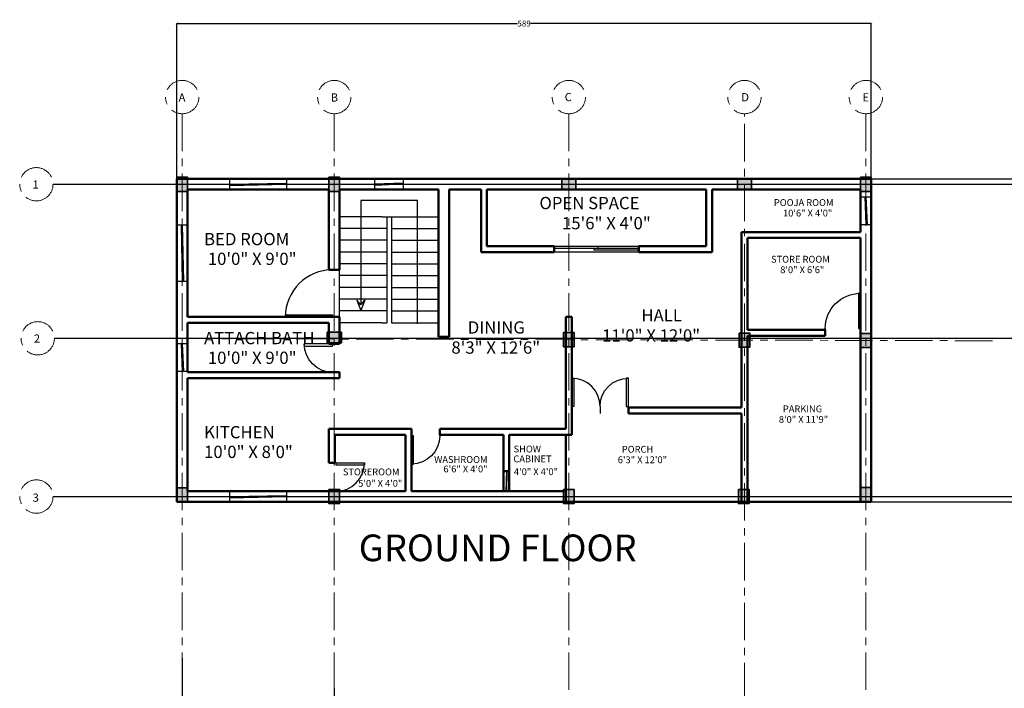
# Model space of a CAD drawing. Units: inches. Extents: x 1455 to 5994, y -182 to 2370.
# Tile 3 of 8: x 1455 to 2291, y 1803 to 2370. Entities that reach past the tile are written whole.
import ezdxf

# ---------------------------------------------------------------- set-up
doc = ezdxf.new("R2010")
doc.units = ezdxf.units.IN
doc.header["$MEASUREMENT"] = 0
doc.linetypes.add('CENTER', pattern=[50.8, 31.75, -6.35, 6.35, -6.35])
for name, color, linetype, lineweight in [('A-ANNO-DIMS', 2, 'Continuous', 18), ('A-ANNO-TEXT', 7, 'Continuous', 25), ('A-AREA-IDEN', 7, 'Continuous', 18), ('A-COLS', 7, 'Continuous', 35), ('A-COLS-PATT', 8, 'Continuous', 13), ('A-DOOR', 5, 'Continuous', 25), ('A-FLOR-STRS', 3, 'Continuous', 25), ('A-GLAZ', 4, 'Continuous', 25), ('A-GRID', 8, 'CENTER', 18), ('A-WALL', 7, 'Continuous', 50)]:
    doc.layers.add(name, color=color, linetype=linetype, lineweight=lineweight)
doc.styles.get("Standard").update_dxf_attribs({"font": 'arial.ttf'})
doc.dimstyles.get("Standard").update_dxf_attribs({"dimtxt": 5, "dimasz": 2, "dimexe": 0.18, "dimexo": 0.0625, "dimgap": 0.09, "dimtad": 0, "dimtih": 1, "dimtoh": 1, "dimdec": 1, "dimzin": 0, "dimdsep": 46, "dimlunit": 3, "dimtxsty": 'Standard', "dimblk": 'ARCHTICK', "dimcen": 0.09, "dimadec": 0, "dimazin": 0, "dimtfac": 1, "dimtdec": 1, "dimtofl": 0, "dimtmove": 0, "dimatfit": 3, "dimfxl": 1, "dimtolj": 1, "dimtzin": 0, "dimarcsym": 0})

# ---------------------------------------------------------------- blocks, each defined once
blk = doc.blocks.new('*U3')
for p, q in [((0, 0), (0, -6)), ((24, 0), (24, -6))]:
    blk.add_line(p, q)
blk.add_lwpolyline([(0, 0), (0, 24), (1.75, 24), (1.75, 0)], close=True)
blk.add_arc((0, 0), 24, 0, 90)
blk = doc.blocks.new('*U4')
for p, q in [((0, 0), (0, -6)), ((40, 0), (40, -6))]:
    blk.add_line(p, q)
blk.add_lwpolyline([(0, 0), (0, 40), (1.75, 40), (1.75, 0)], close=True)
blk.add_arc((0, 0), 40, 0, 90)
blk = doc.blocks.new('*U5')
for p, q in [((0, 0), (0, -6)), ((30, 0), (30, -6))]:
    blk.add_line(p, q)
blk.add_lwpolyline([(0, 0), (0, 30), (1.75, 30), (1.75, 0)], close=True)
blk.add_arc((0, 0), 30, 0, 90)
blk = doc.blocks.new('DOOR-SLIDING')
for p, q in [((0, 2.96), (37.51, 2.96)), ((34.07, 1.25), (34.07, 2.97)), ((72, 1.25), (34.07, 1.25)), ((37.51, 2.96), (37.51, 4.69)), ((37.51, 2.96), (72, 2.96))]:
    blk.add_line(p, q)
blk.add_lwpolyline([(0, 4.69), (72, 4.69), (72, -0.31), (0, -0.31)], close=True)
blk = doc.blocks.new('WIN-600')
for p, q in [((0, 0), (0, 24)), ((0.5, 0), (0.5, 24)), ((1, 0), (1, 24))]:
    blk.add_line(p, q)
blk = doc.blocks.new('WIN-1200')
for p, q in [((0, 1), (48, 1)), ((0, 0.5), (48, 0.5)), ((0, 0), (48, 0))]:
    blk.add_line(p, q)
blk = doc.blocks.new('WIN-450')
for p, q in [((0, 17), (0, 0)), ((0.2, 17), (0.2, 0)), ((0.4, 17), (0.4, 0))]:
    blk.add_line(p, q)
blk = doc.blocks.new('_ArchTick')
at = {"color": 0, "linetype": 'ByBlock', "const_width": 0.15}
blk.add_lwpolyline([(-0.5, -0.5), (0.5, 0.5)], dxfattribs=at)
blk = doc.blocks.new('*D35')
at = {"layer": 'A-ANNO-DIMS', "color": 0, "lineweight": -2, "transparency": 16777216}
for p, q in [((1593.29, 1828.67), (1593.29, 1744.59)), ((1722.29, 1802.99), (1722.29, 1744.59)), ((1593.29, 1744.77), (1652.41, 1744.77)), ((1722.29, 1744.77), (1663.18, 1744.77))]:
    blk.add_line(p, q, dxfattribs=at)
at = {"layer": 'Defpoints', "color": 0, "lineweight": 25, "transparency": 16777216}
for p in [(1593.29, 1828.73), (1722.29, 1803.05), (1722.29, 1744.77)]:
    blk.add_point(p, dxfattribs=at)
at = {"layer": 'A-ANNO-DIMS', "color": 0, "lineweight": -2, "transparency": 16777216, "xscale": 2, "yscale": 2, "zscale": 2, "rotation": 180}
blk.add_blockref('_ArchTick', (1593.29, 1744.77), dxfattribs=at)
at = {"layer": 'A-ANNO-DIMS', "color": 0, "lineweight": -2, "transparency": 16777216, "xscale": 2, "yscale": 2, "zscale": 2}
blk.add_blockref('_ArchTick', (1722.29, 1744.77), dxfattribs=at)
at = {"layer": 'A-ANNO-DIMS', "color": 0, "transparency": 16777216, "insert": (1657.79, 1744.77), "char_height": 5, "attachment_point": 5}
blk.add_mtext('\\A1;129', dxfattribs=at)
blk = doc.blocks.new('*D39')
at = {"layer": 'A-ANNO-DIMS', "color": 0, "lineweight": -2, "transparency": 16777216}
for p, q in [((1483.73, 2230.77), (2434.6, 2230.77)), ((2434.42, 2230.77), (2434.42, 2168.07)), ((2434.42, 2100.07), (2434.42, 2162.78)), ((1484.89, 2100.07), (2434.6, 2100.07))]:
    blk.add_line(p, q, dxfattribs=at)
at = {"layer": 'Defpoints', "color": 0, "lineweight": 25, "transparency": 16777216}
for p in [(1483.66, 2230.77), (1484.83, 2100.07), (2434.42, 2100.07)]:
    blk.add_point(p, dxfattribs=at)
at = {"layer": 'A-ANNO-DIMS', "color": 0, "lineweight": -2, "transparency": 16777216, "xscale": 2, "yscale": 2, "zscale": 2}
for p, rotation in [((2434.42, 2230.77), 90), ((2434.42, 2100.07), 270)]:
    blk.add_blockref('_ArchTick', p, dxfattribs=dict(at, rotation=rotation))
at = {"layer": 'A-ANNO-DIMS', "color": 0, "transparency": 16777216, "insert": (2434.42, 2165.42), "char_height": 5, "attachment_point": 5}
blk.add_mtext('\\A1;130.7', dxfattribs=at)
blk = doc.blocks.new('*D40')
at = {"layer": 'A-ANNO-DIMS', "color": 0, "lineweight": -2, "transparency": 16777216}
for p, q in [((1484.89, 2100.07), (2434.6, 2100.07)), ((2434.42, 2100.07), (2434.42, 2035.57)), ((2434.42, 1965.77), (2434.42, 2030.28)), ((1483.73, 1965.77), (2434.6, 1965.77))]:
    blk.add_line(p, q, dxfattribs=at)
at = {"layer": 'Defpoints', "color": 0, "lineweight": 25, "transparency": 16777216}
for p in [(1484.83, 2100.07), (1483.66, 1965.77), (2434.42, 1965.77)]:
    blk.add_point(p, dxfattribs=at)
at = {"layer": 'A-ANNO-DIMS', "color": 0, "lineweight": -2, "transparency": 16777216, "xscale": 2, "yscale": 2, "zscale": 2}
for p, rotation in [((2434.42, 2100.07), 90), ((2434.42, 1965.77), 270)]:
    blk.add_blockref('_ArchTick', p, dxfattribs=dict(at, rotation=rotation))
at = {"layer": 'A-ANNO-DIMS', "color": 0, "transparency": 16777216, "insert": (2434.42, 2032.92), "char_height": 5, "attachment_point": 5}
blk.add_mtext('\\A1;134.3', dxfattribs=at)
blk = doc.blocks.new('*D41')
at = {"layer": 'A-ANNO-DIMS', "color": 0, "lineweight": -2, "transparency": 16777216}
for p, q in [((1588.79, 2235.34), (1588.79, 2367.36)), ((1588.79, 2367.18), (1877.68, 2367.18)), ((2177.79, 2367.18), (1888.91, 2367.18)), ((2177.79, 2235.34), (2177.79, 2367.36))]:
    blk.add_line(p, q, dxfattribs=at)
at = {"layer": 'Defpoints', "color": 0, "lineweight": 25, "transparency": 16777216}
for p in [(2177.79, 2367.18), (1588.79, 2235.27), (2177.79, 2235.27)]:
    blk.add_point(p, dxfattribs=at)
at = {"layer": 'A-ANNO-DIMS', "color": 0, "lineweight": -2, "transparency": 16777216, "xscale": 2, "yscale": 2, "zscale": 2, "rotation": 180}
blk.add_blockref('_ArchTick', (1588.79, 2367.18), dxfattribs=at)
at = {"layer": 'A-ANNO-DIMS', "color": 0, "lineweight": -2, "transparency": 16777216, "xscale": 2, "yscale": 2, "zscale": 2}
blk.add_blockref('_ArchTick', (2177.79, 2367.18), dxfattribs=at)
at = {"layer": 'A-ANNO-DIMS', "color": 0, "transparency": 16777216, "insert": (1883.29, 2367.18), "char_height": 5, "attachment_point": 5}
blk.add_mtext('\\A1;589', dxfattribs=at)
blk = doc.blocks.new('*D42')
at = {"layer": 'A-ANNO-DIMS', "color": 0, "lineweight": -2, "transparency": 16777216}
for p, q in [((2177.86, 2235.27), (2434.6, 2235.27)), ((2434.42, 2235.27), (2434.42, 2100.96)), ((2434.42, 1961.36), (2434.42, 2095.67)), ((2177.86, 1961.36), (2434.6, 1961.36))]:
    blk.add_line(p, q, dxfattribs=at)
at = {"layer": 'Defpoints', "color": 0, "lineweight": 25, "transparency": 16777216}
for p in [(2177.79, 2235.27), (2434.42, 2235.27), (2177.79, 1961.36)]:
    blk.add_point(p, dxfattribs=at)
at = {"layer": 'A-ANNO-DIMS', "color": 0, "lineweight": -2, "transparency": 16777216, "xscale": 2, "yscale": 2, "zscale": 2}
for p, rotation in [((2434.42, 2235.27), 90), ((2434.42, 1961.36), 270)]:
    blk.add_blockref('_ArchTick', p, dxfattribs=dict(at, rotation=rotation))
at = {"layer": 'A-ANNO-DIMS', "color": 0, "transparency": 16777216, "insert": (2434.42, 2098.32), "char_height": 5, "attachment_point": 5}
blk.add_mtext('\\A1;273.9', dxfattribs=at)

msp = doc.modelspace()

# ---------------------------------------------------------------- hatches: boundary and pattern name
at = {"layer": 'A-COLS-PATT'}
h = msp.add_hatch(color=256, dxfattribs=at)
h.dxf.hatch_style = 1
h.paths.add_polyline_path([(1597.7942, 2236.774), (1588.7942, 2236.774), (1588.7942, 2224.774), (1597.7942, 2224.774)])
h = msp.add_hatch(color=256, dxfattribs=at)
h.dxf.hatch_style = 1
h.paths.add_polyline_path([(1726.7942, 2236.774), (1717.7942, 2236.774), (1717.7942, 2224.774), (1726.7942, 2224.774)])
h = msp.add_hatch(color=256, dxfattribs=at)
h.dxf.hatch_style = 1
h.paths.add_polyline_path([(1915.2942, 2235.274), (1915.2942, 2226.274), (1927.2942, 2226.274), (1927.2942, 2235.274)])
h = msp.add_hatch(color=256, dxfattribs=at)
h.dxf.hatch_style = 1
h.paths.add_polyline_path([(2064.2942, 2235.274), (2064.2942, 2226.274), (2076.2942, 2226.274), (2076.2942, 2235.274)])
h = msp.add_hatch(color=256, dxfattribs=at)
h.dxf.hatch_style = 1
h.paths.add_polyline_path([(2177.7942, 2236.774), (2168.7942, 2236.774), (2168.7942, 2224.774), (2177.7942, 2224.774)])
h = msp.add_hatch(color=256, dxfattribs=at)
h.dxf.hatch_style = 1
h.paths.add_polyline_path([(1716.2942, 2105.179), (1716.2942, 2096.179), (1728.2942, 2096.179), (1728.2942, 2105.179)])
h = msp.add_hatch(color=256, dxfattribs=at)
h.dxf.hatch_style = 1
h.paths.add_polyline_path([(1925.7942, 2104.9263), (1916.7942, 2104.9263), (1916.7942, 2092.9263), (1925.7942, 2092.9263)])
h = msp.add_hatch(color=256, dxfattribs=at)
h.dxf.hatch_style = 1
h.paths.add_polyline_path([(2074.7942, 2104.537), (2065.7942, 2104.537), (2065.7942, 2092.537), (2074.7942, 2092.537)])
h = msp.add_hatch(color=256, dxfattribs=at)
h.dxf.hatch_style = 1
h.paths.add_polyline_path([(2177.7942, 2104.2678), (2168.7942, 2104.2678), (2168.7942, 2092.2678), (2177.7942, 2092.2678)])
h = msp.add_hatch(color=256, dxfattribs=at)
h.dxf.hatch_style = 1
h.paths.add_polyline_path([(1597.7942, 1973.1902), (1588.7942, 1973.1902), (1588.7942, 1961.1902), (1597.7942, 1961.1902)])
h = msp.add_hatch(color=256, dxfattribs=at)
h.dxf.hatch_style = 1
h.paths.add_polyline_path([(1726.7942, 1971.774), (1717.7942, 1971.774), (1717.7942, 1959.774), (1726.7942, 1959.774)])
h = msp.add_hatch(color=256, dxfattribs=at)
h.dxf.hatch_style = 1
h.paths.add_polyline_path([(1925.7942, 1971.774), (1916.7942, 1971.774), (1916.7942, 1959.774), (1925.7942, 1959.774)])
h = msp.add_hatch(color=256, dxfattribs=at)
h.dxf.hatch_style = 1
h.paths.add_polyline_path([(2074.1779, 1971.774), (2065.1779, 1971.774), (2065.1779, 1959.774), (2074.1779, 1959.774)])
h = msp.add_hatch(color=256, dxfattribs=at)
h.dxf.hatch_style = 1
h.paths.add_polyline_path([(2177.7942, 1973.3596), (2168.7942, 1973.3596), (2168.7942, 1961.3596), (2177.7942, 1961.3596)])

# ---------------------------------------------------------------- linework, layer by layer
at = {"layer": 'A-COLS'}
for points in [[(1588.7942, 2236.774), (1597.7942, 2236.774), (1597.7942, 2224.774), (1588.7942, 2224.774)], [(1717.7942, 2236.774), (1726.7942, 2236.774), (1726.7942, 2224.774), (1717.7942, 2224.774)], [(1915.2942, 2226.274), (1915.2942, 2235.274), (1927.2942, 2235.274), (1927.2942, 2226.274)], [(2064.2942, 2226.274), (2064.2942, 2235.274), (2076.2942, 2235.274), (2076.2942, 2226.274)], [(2168.7942, 2236.774), (2177.7942, 2236.774), (2177.7942, 2224.774), (2168.7942, 2224.774)], [(1716.2942, 2096.179), (1716.2942, 2105.179), (1728.2942, 2105.179), (1728.2942, 2096.179)], [(1916.7942, 2104.9263), (1925.7942, 2104.9263), (1925.7942, 2092.9263), (1916.7942, 2092.9263)], [(2065.7942, 2104.537), (2074.7942, 2104.537), (2074.7942, 2092.537), (2065.7942, 2092.537)], [(2168.7942, 2104.2678), (2177.7942, 2104.2678), (2177.7942, 2092.2678), (2168.7942, 2092.2678)], [(1588.7942, 1973.1902), (1597.7942, 1973.1902), (1597.7942, 1961.1902), (1588.7942, 1961.1902)], [(1717.7942, 1971.774), (1726.7942, 1971.774), (1726.7942, 1959.774), (1717.7942, 1959.774)], [(1916.7942, 1971.774), (1925.7942, 1971.774), (1925.7942, 1959.774), (1916.7942, 1959.774)], [(2065.1779, 1971.774), (2074.1779, 1971.774), (2074.1779, 1959.774), (2065.1779, 1959.774)], [(2168.7942, 1973.3596), (2177.7942, 1973.3596), (2177.7942, 1961.3596), (2168.7942, 1961.3596)]]:
    msp.add_lwpolyline(points, close=True, dxfattribs=at)
at = {"layer": 'A-FLOR-STRS'}
for p, q in [((1792.7942, 2217.1453), (1744.7942, 2217.1453)), ((1744.7942, 2217.1453), (1744.7942, 2128.5876)), ((1792.7942, 2112.4497), (1792.7942, 2217.1453)), ((1762.7942, 2203.274), (1726.7942, 2203.274)), ((1762.7942, 2203.274), (1774.7942, 2203.274)), ((1766.7942, 2203.274), (1766.7942, 2113.274)), ((1770.7942, 2203.274), (1770.7942, 2113.274)), ((1774.7942, 2203.274), (1810.7942, 2203.274)), ((1766.7942, 2193.274), (1726.7942, 2193.274)), ((1770.7942, 2193.274), (1810.7942, 2193.274)), ((1766.7942, 2183.274), (1726.7942, 2183.274)), ((1770.7942, 2183.274), (1810.7942, 2183.274)), ((1766.7942, 2173.274), (1726.7942, 2173.274)), ((1770.7942, 2173.274), (1810.7942, 2173.274)), ((1766.7942, 2163.274), (1726.7942, 2163.274)), ((1726.7942, 2113.274), (1726.7942, 2160.274)), ((1770.7942, 2163.274), (1810.7942, 2163.274)), ((1766.7942, 2153.274), (1726.7942, 2153.274)), ((1770.7942, 2153.274), (1810.7942, 2153.274)), ((1766.7942, 2143.274), (1726.7942, 2143.274)), ((1770.7942, 2143.274), (1810.7942, 2143.274)), ((1766.7942, 2133.274), (1726.7942, 2133.274)), ((1744.7942, 2128.5876), (1741.4465, 2132.4497)), ((1741.4465, 2132.4497), (1744.7942, 2123.5688)), ((1744.7942, 2128.5876), (1748.1419, 2132.4497)), ((1748.1419, 2132.4497), (1744.7942, 2123.5688)), ((1770.7942, 2133.274), (1810.7942, 2133.274)), ((1766.7942, 2123.274), (1726.7942, 2123.274)), ((1770.7942, 2123.274), (1810.7942, 2123.274)), ((1762.7942, 2113.274), (1726.7942, 2113.274)), ((1762.7942, 2113.274), (1766.7942, 2113.274)), ((1770.7942, 2113.274), (1774.7942, 2113.274)), ((1774.7942, 2113.274), (1810.7942, 2113.274))]:
    msp.add_line(p, q, dxfattribs=at)
at = {"layer": 'A-GLAZ'}
for points in [[(1633.7942, 2235.274), (1681.7942, 2235.274), (1681.7942, 2226.274), (1633.7942, 2226.274)], [(1756.7942, 2235.274), (1780.7942, 2235.274), (1780.7942, 2226.274), (1756.7942, 2226.274)], [(2168.7942, 2196.274), (2168.7942, 2220.274), (2177.7942, 2220.274), (2177.7942, 2196.274)], [(1597.7942, 2196.274), (1597.7942, 2148.274), (1588.7942, 2148.274), (1588.7942, 2196.274)], [(1588.7942, 2071.7739), (1588.7942, 2095.7739), (1597.7942, 2095.7739), (1597.7942, 2071.7739)], [(1870.7942, 1970.274), (1865.7942, 1970.274), (1865.7942, 1987.274), (1870.7942, 1987.274)], [(1633.7942, 1970.274), (1681.7942, 1970.274), (1681.7942, 1961.274), (1633.7942, 1961.274)]]:
    msp.add_lwpolyline(points, close=True, dxfattribs=at)
at = {"layer": 'A-GRID'}
for p, q in [((1593.2942, 2290.6569), (1593.2942, 1828.7288)), ((1722.2942, 2290.6569), (1722.2942, 1803.0507)), ((1921.2942, 2290.6569), (1921.2942, 1801.7341)), ((2070.2942, 1793.0189), (2070.2942, 2290.6569)), ((2173.2942, 2290.6569), (2173.2942, 1794.3991)), ((1483.6636, 2230.774), (2284.5122, 2230.774)), ((2280.5998, 2097.9874), (1484.8312, 2100.0669)), ((1483.6636, 1965.774), (2386.1674, 1965.774))]:
    msp.add_line(p, q, dxfattribs=at)
for centre in [(1593.2942, 2304.7952), (1722.2942, 2304.7952), (1921.2942, 2304.7952), (2070.2942, 2304.7952), (2173.2942, 2304.7952), (1469.5253, 2230.774), (1470.6929, 2100.0669), (1469.5253, 1965.774)]:
    msp.add_circle(centre, 14.1383, dxfattribs=at)
at = {"layer": 'A-WALL'}
for p, q in [((1588.7942, 2235.274), (1588.7942, 1961.274)), ((1588.7942, 2235.274), (2177.7942, 2235.274)), ((2177.7942, 2235.274), (2177.7942, 1961.274)), ((1597.7942, 2226.274), (1597.7942, 2118.274)), ((1597.7942, 2226.274), (1717.7942, 2226.274)), ((1717.7942, 2226.274), (1717.7942, 2158.1614)), ((1726.7942, 2226.274), (1726.7942, 2158.274)), ((1726.7942, 2226.274), (1810.7942, 2226.274)), ((1810.7942, 2226.274), (1810.7942, 2101.2917)), ((1819.7942, 2226.274), (1819.7942, 2101.2917)), ((1819.7942, 2226.274), (1846.7942, 2226.274)), ((1846.7942, 2226.274), (1846.7942, 2190.274)), ((1851.7942, 2226.274), (1851.7942, 2190.274)), ((1851.7942, 2226.274), (2037.7942, 2226.274)), ((2037.7942, 2226.274), (2037.7942, 2178.274)), ((2042.7942, 2226.274), (2042.7942, 2190.274)), ((2042.7942, 2226.274), (2067.7942, 2226.274)), ((2067.7942, 2226.274), (2168.7942, 2226.274)), ((2168.7942, 2226.274), (2168.7942, 2190.274)), ((1846.7942, 2190.274), (1846.7942, 2173.274)), ((1851.7942, 2190.274), (1851.7942, 2178.274)), ((2042.7942, 2190.274), (2042.7942, 2173.274)), ((2067.7942, 2190.274), (2067.7942, 2041.274)), ((2067.7942, 2190.274), (2168.7942, 2190.274)), ((2072.7942, 2185.274), (2072.7942, 2107.274)), ((2072.7942, 2185.274), (2168.7942, 2185.274)), ((2168.7942, 2185.274), (2168.7942, 2119.274)), ((1846.7942, 2173.274), (1908.7942, 2173.274)), ((1851.7942, 2178.274), (1908.7942, 2178.274)), ((1908.7942, 2178.274), (1908.7942, 2173.274)), ((1980.7942, 2178.274), (2037.7942, 2178.274)), ((1980.7942, 2178.274), (1980.7942, 2173.274)), ((1980.7942, 2173.274), (2042.7942, 2173.274)), ((1717.7942, 2158.1614), (1726.7942, 2158.274)), ((1597.7942, 2118.274), (1717.7942, 2118.274)), ((1717.7942, 2118.274), (1726.7942, 2118.274)), ((1726.7942, 2118.274), (1726.7942, 2113.274)), ((1918.7942, 2118.274), (1918.7942, 2023.274)), ((1918.7942, 2118.274), (1923.7942, 2118.274)), ((1923.7942, 2118.274), (1923.7942, 2041.274)), ((2168.7942, 2119.274), (2168.7942, 2107.274)), ((1597.7942, 2113.274), (1597.7942, 2071.274)), ((1597.7942, 2113.274), (1717.7942, 2113.274)), ((1717.7942, 2113.274), (1717.7942, 2095.274)), ((1726.7942, 2113.274), (1726.7942, 2095.274)), ((2072.7942, 2107.274), (2138.7942, 2107.274)), ((2138.7942, 2107.274), (2138.7942, 2102.274)), ((2168.7942, 2107.274), (2168.7942, 2102.274)), ((1819.7942, 2101.2917), (1810.7942, 2101.2917)), ((2072.7942, 2102.274), (2072.7942, 1961.274)), ((2072.7942, 2102.274), (2138.7942, 2102.274)), ((2168.7942, 2102.274), (2168.7942, 1961.274)), ((1717.7942, 2095.274), (1726.7942, 2095.274)), ((1597.7942, 2071.274), (1717.7942, 2071.274)), ((1597.7942, 2066.274), (1597.7942, 1970.274)), ((1597.7942, 2066.274), (1726.7942, 2066.274)), ((1717.7942, 2071.274), (1726.7942, 2071.274)), ((1726.7942, 2071.274), (1726.7942, 2066.274)), ((1923.7942, 2041.274), (1923.7942, 2036.274)), ((1971.7942, 2041.274), (2067.7942, 2041.274)), ((1971.7942, 2041.274), (1971.7942, 2036.274)), ((1923.7942, 2036.274), (1923.7942, 2018.274)), ((1971.7942, 2036.274), (2067.7942, 2036.274)), ((2067.7942, 2036.274), (2067.7942, 1961.274)), ((1717.7942, 2023.274), (1717.7942, 1994.274)), ((1717.7942, 2023.274), (1787.7942, 2023.274)), ((1787.7942, 2018.274), (1787.7942, 2023.274)), ((1811.7942, 2023.274), (1918.7942, 2023.274)), ((1811.7942, 2018.274), (1811.7942, 2023.274)), ((1722.7942, 2018.274), (1722.7942, 1994.274)), ((1722.7942, 2018.274), (1782.7942, 2018.274)), ((1782.7942, 2018.274), (1782.7942, 1970.274)), ((1787.7942, 2018.274), (1787.7942, 1970.274)), ((1811.7942, 2018.274), (1865.7942, 2018.274)), ((1865.7942, 2018.274), (1865.7942, 1970.274)), ((1870.7942, 2018.274), (1870.7942, 1970.274)), ((1870.7942, 2018.274), (1923.7942, 2018.274)), ((1918.7942, 2018.274), (1918.7942, 1961.274)), ((1717.7942, 1994.274), (1722.7942, 1994.274)), ((1865.7942, 1987.274), (1870.7942, 1987.274)), ((1597.7942, 1970.274), (1717.7942, 1970.274)), ((1717.7942, 1970.274), (1722.7942, 1970.274)), ((1722.7942, 1970.274), (1782.7942, 1970.274)), ((1775.7942, 1970.274), (1782.7942, 1970.274)), ((1787.7942, 1970.274), (1865.7942, 1970.274)), ((1865.7942, 1970.274), (1870.7942, 1970.274)), ((1870.7942, 1970.274), (1918.7942, 1970.274)), ((1588.7942, 1961.274), (2072.7942, 1961.274)), ((2072.7942, 1961.274), (2177.7942, 1961.274))]:
    msp.add_line(p, q, dxfattribs=at)

# ---------------------------------------------------------------- block references
at = {"layer": 'A-DOOR'}
for name, p in [('DOOR-SLIDING', (1908.7947, 2173.588)), ('*U3', (1923.7942, 2042.274))]:
    msp.add_blockref(name, p, dxfattribs=at)
for name, p, rotation in [('*U4', (1720.7942, 2118.274), 90.00000000000003), ('*U3', (1723.7942, 1994.274), 270)]:
    msp.add_blockref(name, p, dxfattribs=dict(at, rotation=rotation))
at = {"layer": 'A-DOOR', "xscale": -1}
for name, p in [('*U5', (2168.7942, 2108.274)), ('*U3', (1971.7942, 2042.274))]:
    msp.add_blockref(name, p, dxfattribs=at)
for p, rotation in [((1720.7942, 2095.274), 90), ((1787.7942, 2017.274), 180)]:
    msp.add_blockref('*U3', p, dxfattribs=dict(at, rotation=rotation))
at = {"layer": 'A-GLAZ'}
for name, p, rotation in [('WIN-1200', (1633.8103, 2229.7742), 1.193489423981132), ('WIN-600', (1780.8047, 2230.7745), 92.3859440303866), ('WIN-600', (2173.2937, 2220.2845), 182.3859440303908), ('WIN-1200', (1592.2943, 2196.258), 271.1934894239826), ('WIN-600', (1593.2937, 2095.7844), 182.3859440303887), ('WIN-450', (1867.8948, 1970.281), 358.6521127197998), ('WIN-1200', (1633.8103, 1964.7742), 1.193489423981132)]:
    msp.add_blockref(name, p, dxfattribs=dict(at, rotation=rotation))

# ---------------------------------------------------------------- texts
at = {"layer": 'A-ANNO-TEXT'}
msp.add_text('GROUND FLOOR', height=22.629125, dxfattribs=at).set_placement((1743.0603, 1910.9233))
at = {"layer": 'A-AREA-IDEN'}
for s, height, p in [('OPEN SPACE', 10.41336, (1896.3245, 2209.6581)), ('POOJA ROOM', 5.78042, (2095.256, 2212.3782)), ('10\'6" X 4\'0"', 5.780423, (2103.0133, 2203.4494)), ('15\'6" X 4\'0"', 10.413361, (1915.4777, 2192.5903)), ('BED ROOM ', 10.41336, (1611.8145, 2179.0544)), (' 10\'0" X 9\'0"', 10.413361, (1611.8145, 2162.3263)), ('STORE ROOM', 5.78042, (2092.8684, 2164.2915)), ('8\'0" X 6\'6"', 5.780423, (2100.6257, 2155.3627)), ('HALL', 10.41336, (1982.8659, 2114.35)), ('DINING', 10.41336, (1835.5459, 2104.0757)), ('ATTACH BATH', 10.413361, (1611.8145, 2095.0591)), ('11\'0" X 12\'0"', 10.413361, (1949.5084, 2097.2822)), ('8\'3" X 12\'6"', 10.413361, (1821.6551, 2087.0079)), (' 10\'0" X 9\'0"', 10.413361, (1611.8145, 2078.331)), ('PARKING', 5.78042, (2102.8747, 2037.3018)), ('8\'0" X 11\'9"', 5.780423, (2099.4734, 2028.373)), ('KITCHEN', 10.41336, (1611.8145, 2015.2101)), ('10\'0" X 8\'0"', 10.413361, (1611.8145, 1998.482)), ('SHOW ', 5.78042, (1874.4324, 2003.2325)), ('PORCH', 5.78042, (1966.212, 2003.0215)), ('WASHROOM', 5.78042, (1807.0544, 1994.3176)), ('CABINET', 5.78042, (1874.226, 1994.8806)), ('6\'3" X 12\'0"', 5.780423, (1962.8107, 1994.0927)), ('STOREROOM', 5.78042, (1729.5513, 1983.8092)), ('6\'6" X 4\'0"', 5.780423, (1814.9143, 1986.2887)), ('4\'0" X 4\'0"', 5.780423, (1874.6931, 1983.9796)), ('5\'0" X 4\'0"', 5.780423, (1742.5915, 1974.0612))]:
    msp.add_text(s, height=height, dxfattribs=at).set_placement(p)
at = {"layer": 'A-GRID'}
for s, p in [('A', (1590.2053, 2300.9515)), ('B', (1719.275, 2300.9515)), ('C', (1917.7661, 2301.3327)), ('D', (2067.6005, 2301.179)), ('E', (2170.3878, 2301.0448)), ('1', (1466.2547, 2227.0875)), ('2', (1467.4223, 2096.3803)), ('3', (1466.3802, 1961.371))]:
    msp.add_text(s, height=6.963, dxfattribs=at).set_placement(p)

# ---------------------------------------------------------------- dimensions: what is measured, and where the dimension line sits
at = {"layer": 'A-ANNO-DIMS'}
for base, p1, p2, picture, middle in [((2177.7942, 2367.1835), (1588.7942, 2235.274), (2177.7942, 2235.274), '*D41', (1883.2942, 2367.1835)), ((1722.2942, 1744.7689), (1593.2942, 1828.7288), (1722.2942, 1803.0507), '*D35', (1657.7942, 1744.7689))]:
    dim = msp.add_linear_dim(base=base, p1=p1, p2=p2, dimstyle='Standard', override={"dimdec": 0, "dimlfac": 1, "dimrnd": 0, "dimzin": 0, "dimdsep": 46, "dimlunit": 2}, dxfattribs=at)
    dim.commit()
    dim.dimension.update_dxf_attribs({"geometry": picture, "text_midpoint": middle})
for base, p1, p2, picture, middle in [((2434.4174, 2100.0669), (1483.6636, 2230.774), (1484.8312, 2100.0669), '*D39', (2434.4174, 2165.4205)), ((2434.4174, 2235.274), (2177.7942, 1961.3596), (2177.7942, 2235.274), '*D42', (2434.4174, 2098.3168)), ((2434.4174, 1965.774), (1484.8312, 2100.0669), (1483.6636, 1965.774), '*D40', (2434.4174, 2032.9205))]:
    dim = msp.add_linear_dim(base=base, p1=p1, p2=p2, angle=90, dimstyle='Standard', override={"dimdec": 1, "dimlfac": 1, "dimrnd": 0, "dimzin": 0, "dimdsep": 46, "dimlunit": 2}, dxfattribs=at)
    dim.commit()
    dim.dimension.update_dxf_attribs({"geometry": picture, "text_midpoint": middle})

doc.saveas('drawing.dxf')
